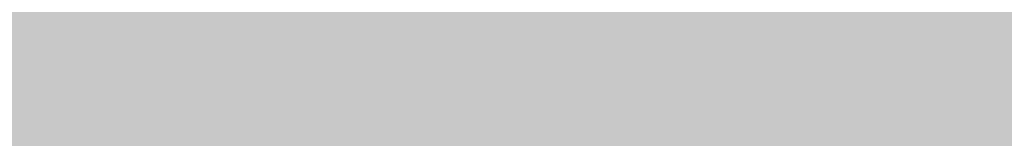
# Model space of a CAD drawing. Units: inches. Extents: x 2083 to 3317, y 1141 to 2115.
# Tile 134 of 256: x 3123.979 to 3126.132, y 1263.355 to 1263.613. Entities that reach past the tile are written whole.
import ezdxf

# ---------------------------------------------------------------- set-up
doc = ezdxf.new("R2010")
doc.units = ezdxf.units.IN
doc.layers.add('A-ANNO-DIMS', color=2, linetype='Continuous', lineweight=18)
doc.layers.add('A-WALL-PATT', color=251, linetype='Continuous', lineweight=13, true_color=0x636466)
doc.styles.get("Standard").update_dxf_attribs({"font": 'arial.ttf'})
doc.dimstyles.new('ISO-25', dxfattribs={"dimtxt": 12, "dimasz": 12, "dimexe": 1.25, "dimexo": 0.625, "dimtad": 1, "dimlunit": 3, "dimtxsty": 'Standard', "dimcen": 2.5, "dimadec": 0, "dimazin": 0, "dimtfac": 1, "dimtmove": 0, "dimatfit": 3, "dimfxl": 1, "dimarcsym": 0})

# ---------------------------------------------------------------- blocks, each defined once
blk = doc.blocks.new('*D26')
at = {"layer": 'A-ANNO-DIMS', "color": 0, "lineweight": -2, "transparency": 16777216}
for p, q in [((3088.9858, 1274.9151), (3088.9858, 1270.952)), ((3111.24, 1274.9151), (3111.24, 1270.952)), ((3076.9858, 1272.202), (2840.2624, 1272.202)), ((3111.24, 1272.202), (3088.9858, 1272.202)), ((3123.24, 1272.202), (3135.24, 1272.202))]:
    blk.add_line(p, q, dxfattribs=at)
at = {"layer": 'A-ANNO-DIMS', "color": 0, "transparency": 16777216}
for points in [[(3076.9858, 1274.202), (3076.9858, 1270.202), (3088.9858, 1272.202)], [(3123.24, 1274.202), (3123.24, 1270.202), (3111.24, 1272.202)]]:
    blk.add_solid(points, dxfattribs=at)
at = {"layer": 'Defpoints', "color": 0, "transparency": 16777216}
for p in [(3088.9858, 1275.5401), (3111.24, 1275.5401), (3088.9858, 1272.202)]:
    blk.add_point(p, dxfattribs=at)
at = {"layer": 'A-ANNO-DIMS', "color": 0, "transparency": 16777216, "insert": (2952.6241, 1279.0316), "char_height": 12, "attachment_point": 5}
blk.add_mtext('NIGHTSTAND 1\'-10 1/2" TYP.', dxfattribs=at)
blk = doc.blocks.new('*D27')
at = {"layer": 'A-ANNO-DIMS', "color": 0, "lineweight": -2, "transparency": 16777216}
for p, q in [((3114.5782, 1309.7943), (3114.5782, 1321.7943)), ((3111.865, 1297.7943), (3115.8282, 1297.7943)), ((3114.5782, 1297.7943), (3114.5782, 1275.5401)), ((3111.865, 1275.5401), (3115.8282, 1275.5401)), ((3114.5782, 1263.5401), (3114.5782, 1140.9886))]:
    blk.add_line(p, q, dxfattribs=at)
at = {"layer": 'A-ANNO-DIMS', "color": 0, "transparency": 16777216}
for points in [[(3112.5782, 1309.7943), (3116.5782, 1309.7943), (3114.5782, 1297.7943)], [(3112.5782, 1263.5401), (3116.5782, 1263.5401), (3114.5782, 1275.5401)]]:
    blk.add_solid(points, dxfattribs=at)
at = {"layer": 'Defpoints', "color": 0, "transparency": 16777216}
for p in [(3111.24, 1297.7943), (3111.24, 1275.5401), (3114.5782, 1275.5401)]:
    blk.add_point(p, dxfattribs=at)
at = {"layer": 'A-ANNO-DIMS', "color": 0, "transparency": 16777216, "insert": (3107.7485, 1196.2643), "char_height": 12, "attachment_point": 5, "rotation": 90}
blk.add_mtext('1\'-10 1/2" TYP.', dxfattribs=at)

msp = doc.modelspace()

# ---------------------------------------------------------------- hatches: boundary and pattern name
at = {"layer": 'A-WALL-PATT'}
h = msp.add_hatch(color=256, dxfattribs=at)
h.dxf.hatch_style = 1
h.paths.add_polyline_path([(3126.9598, 2020.7614), (2748.9598, 2020.7614), (2604.9598, 2020.7614), (2226.9598, 2020.7614), (2226.9598, 1702.7614), (2466.9598, 1702.7614), (2466.9598, 1582.7614), (2418.9598, 1582.7614), (2418.9598, 1477.7614), (2226.9598, 1477.7614), (2226.9598, 1263.2614), (2544.9598, 1263.2614), (2544.9598, 1411.7614), (2604.9598, 1411.7614), (2685.9598, 1411.7614), (2685.9598, 1420.7614), (2604.9598, 1420.7614), (2604.9598, 1573.7614), (2604.9598, 1702.7614), (2604.9598, 2011.7614), (2748.9598, 2011.7614), (2748.9598, 1702.7614), (2862.9598, 1702.7614), (2862.9598, 1621.7614), (2871.9598, 1621.7614), (2871.9598, 1702.7614), (2883.9598, 1702.7614), (2883.9598, 1706.9395, -0.026459), (2883.9598, 1711.7614), (2757.9598, 1711.7614), (2757.9598, 1807.7614), (2787.9598, 1807.7614), (2787.9598, 1812.2614), (2757.9598, 1812.2614), (2757.9598, 2011.7614), (2877.9598, 2011.7614), (2877.9598, 1812.2614), (2847.9598, 1812.2614), (2847.9598, 1807.7614), (2889.8357, 1807.7614), (2889.8357, 1812.2614), (2882.4598, 1812.2614), (2882.4598, 2011.7614), (3117.9598, 2011.7614), (3117.9598, 1812.2614), (2937.8357, 1812.2614), (2937.8357, 1807.7614), (2995.7098, 1807.7614), (2995.7098, 1796.1177), (3000.2098, 1796.1177), (3000.2098, 1807.7614), (3117.9598, 1807.7614), (3117.9598, 1711.7614), (3000.2098, 1711.7614), (3000.2098, 1760.1177), (2998.5727, 1760.1177, -0.020711), (2995.7098, 1760.1177), (2995.7098, 1711.7614), (2931.9598, 1711.7614), (2931.9598, 1702.7614), (3126.9598, 1702.7614)])
h.paths.add_polyline_path([(2471.4598, 2011.7614), (2471.4598, 1810.0114), (2462.7169, 1810.0114), (2462.7169, 1805.5114), (2505.9598, 1805.5114), (2505.9598, 1810.0114), (2475.9598, 1810.0114), (2475.9598, 2011.7614), (2595.9598, 2011.7614), (2595.9598, 1810.0114), (2565.9598, 1810.0114), (2565.9598, 1805.5114), (2595.9598, 1805.5114), (2595.9598, 1711.7614), (2235.9598, 1711.7614), (2235.9598, 1805.5114), (2353.7098, 1805.5114), (2353.7098, 1796.0542), (2358.2098, 1796.0542), (2358.2098, 1805.5114), (2414.7169, 1805.5114), (2414.7169, 1810.0114), (2235.9598, 1810.0114), (2235.9598, 2011.7614)], flags=16)
h.paths.add_polyline_path([(2270.2047, 1994.61), (2270.2047, 1970.61), (2246.2047, 1970.61), (2246.2047, 1994.61)], flags=0)
edge = h.paths.add_edge_path(flags=0)
edge.add_ellipse((2332.0274, 1899.7982), major_axis=(-3.043, 3.043), ratio=0.168252, start_angle=-161.3322, end_angle=-156.3071, ccw=False)
edge.add_ellipse((2333.082, 1898.7435), major_axis=(-1.0546, 1.0546), ratio=0.453532, start_angle=-123.371, end_angle=-94.1591)
edge = h.paths.add_edge_path(flags=0)
edge.add_ellipse((2332.0274, 1968.8763), major_axis=(3.043, 3.043), ratio=0.168252, start_angle=18.6678, end_angle=23.6929)
edge.add_spline(control_points=[(2332.9256, 1970.6911), (2332.2268, 1970.3361), (2330.8937, 1969.6589), (2328.4131, 1970.9321), (2327.2039, 1967.7487), (2324.7096, 1969.9556), (2322.5328, 1967.0124), (2320.0128, 1971.2958), (2317.6803, 1968.1578), (2316.0405, 1967.102), (2315.4269, 1966.8096)], knot_values=[0, 0, 0, 0, 2.267059, 4.324559, 6.685584, 8.878641, 11.121502, 14.300359, 17.755284, 19.732645, 19.732645, 19.732645, 19.732645], degree=3, periodic=0)
edge.add_ellipse((2332.0274, 1968.8763), major_axis=(3.043, 3.043), ratio=0.168252, start_angle=18.6678, end_angle=23.6929, ccw=False)
edge.add_ellipse((2333.082, 1969.9309), major_axis=(1.0546, 1.0546), ratio=0.453532, start_angle=56.629, end_angle=85.8409, ccw=False)
edge = h.paths.add_edge_path(flags=0)
edge.add_spline(control_points=[(2296.4283, 1967.9879), (2293.6278, 1965.3363), (2287.7036, 1959.7271), (2299.7439, 1949.9957), (2294.5326, 1935.6685), (2290.5732, 1920.6035), (2293.3941, 1909.9737), (2296.1854, 1904.9665)], knot_values=[0.099185, 0.099185, 0.099185, 0.099185, 0.345301, 0.619822, 0.982653, 1.386093, 1.810555, 1.810555, 1.810555, 1.810555], degree=3, periodic=0)
edge.add_spline(control_points=[(2296.1854, 1904.9665), (2297.3836, 1902.6193), (2298.001, 1901.9493), (2298.553, 1901.4682)], knot_values=[0.006246, 0.006246, 0.006246, 0.006246, 0.055476, 0.055476, 0.055476, 0.055476], degree=3, periodic=0)
edge.add_spline(control_points=[(2298.553, 1901.4682), (2297.2586, 1900.9232), (2295.2253, 1900.2321), (2293.0602, 1900.6142), (2292.1014, 1900.7884), (2292.0896, 1900.7906)], knot_values=[0.312835, 0.312835, 0.312835, 0.312835, 0.40178, 0.474987, 0.475903, 0.475903, 0.475903, 0.475903], degree=3, periodic=0)
edge.add_arc((2292.7936, 1904.6641), 3.937, 215.4209, 259.6982, ccw=False)
edge.add_spline(control_points=[(2289.5853, 1902.3823), (2289.4767, 1902.5351), (2289.3685, 1902.688), (2289.2609, 1902.8412)], knot_values=[0.102872, 0.102872, 0.102872, 0.102872, 0.116896, 0.116896, 0.116896, 0.116896], degree=3, periodic=0)
edge.add_spline(control_points=[(2289.2609, 1902.8412), (2288.6866, 1902.5502), (2287.64, 1902.0199), (2285.8813, 1901.874), (2283.853, 1901.5044), (2281.72, 1899.7105), (2278.467, 1899.4929), (2276.1571, 1901.8832), (2272.259, 1899.8041), (2267.7776, 1901.8432), (2262.2439, 1900.184), (2257.4149, 1901.7821), (2254.3184, 1900.7261), (2253.1783, 1900.3373)], knot_values=[0, 0, 0, 0, 1.907977, 3.477176, 5.261074, 7.972851, 11.680248, 13.717921, 16.939592, 22.789562, 27.502503, 33.595215, 37.145618, 37.145618, 37.145618, 37.145618], degree=3, periodic=0)
edge.add_line((2253.1783, 1900.3373), (2250.2442, 1902.8412))
edge.add_line((2250.2442, 1902.8412), (2250.2442, 1965.8333))
edge.add_line((2250.2442, 1965.8333), (2253.1783, 1968.3371))
edge.add_spline(control_points=[(2253.1783, 1968.3371), (2254.3184, 1967.9483), (2257.4149, 1966.8924), (2262.2439, 1968.4904), (2267.7776, 1966.8313), (2271.5267, 1968.5372), (2273.8759, 1967.8283), (2274.2067, 1967.7276)], knot_values=[0, 0, 0, 0, 0.09018, 0.244935, 0.364644, 0.513233, 0.537855, 0.537855, 0.537855, 0.537855], degree=3, periodic=0)
edge.add_arc((2274.3529, 1963.7933), 3.937, 72.0511, 92.1279, ccw=False)
edge.add_arc((2281.2969, 1985.23), 18.5963, 252.05113, 288.56572)
edge.add_arc((2292.3167, 1956.0289), 12.6461, 71.02679, 113.77822, ccw=False)
edge = h.paths.add_edge_path(flags=0)
edge.add_spline(control_points=[(2274.8994, 1951.8562), (2275.0662, 1951.6166), (2275.2327, 1951.3766), (2275.398, 1951.1359)], knot_values=[1.409916, 1.409916, 1.409916, 1.409916, 1.43159, 1.43159, 1.43159, 1.43159], degree=3, periodic=0)
edge.add_spline(control_points=[(2275.398, 1951.1359), (2275.7921, 1950.5619), (2276.1792, 1949.9838), (2276.5455, 1949.3971)], knot_values=[1.358238, 1.358238, 1.358238, 1.358238, 1.409916, 1.409916, 1.409916, 1.409916], degree=3, periodic=0)
edge.add_line((2276.5455, 1949.3971), (2277.4373, 1947.8622))
edge.add_spline(control_points=[(2277.4373, 1947.8622), (2276.3038, 1945.6731), (2274.6397, 1942.4269), (2274.6316, 1938.0939), (2272.7991, 1930.8515), (2274.3564, 1943.897), (2275.9477, 1947.9234), (2276.5455, 1949.3971)], knot_values=[0.005632, 0.005632, 0.005632, 0.005632, 0.186014, 0.266002, 0.357087, 0.59639, 0.739732, 0.739732, 0.739732, 0.739732], degree=3, periodic=0)
edge.add_spline(control_points=[(2276.5455, 1949.3971), (2276.1792, 1949.9838), (2275.7921, 1950.5619), (2275.398, 1951.1359)], knot_values=[1.358238, 1.358238, 1.358238, 1.358238, 1.409916, 1.409916, 1.409916, 1.409916], degree=3, periodic=0)
edge.add_spline(control_points=[(2275.398, 1951.1359), (2274.9425, 1950.0805), (2274.2078, 1948.0253), (2273.9346, 1944.8515), (2272.4685, 1937.6275), (2273.4662, 1945.6965), (2274.7006, 1951.0595), (2274.8994, 1951.8562)], knot_values=[0.104364, 0.104364, 0.104364, 0.104364, 0.189636, 0.269624, 0.36071, 0.600013, 0.644622, 0.644622, 0.644622, 0.644622], degree=3, periodic=0)
h.paths.add_polyline_path([(2269.1675, 1963.1276, -0.357527), (2268.1706, 1960.9764, -0.092561), (2268.1706, 1939.4363, -0.357527), (2269.1675, 1937.2851, -0.357527), (2267.0163, 1938.282, -0.164785), (2254.6856, 1938.282, -0.357527), (2252.5344, 1937.2851, -0.357527), (2253.5313, 1939.4363, -0.092561), (2253.5313, 1960.9764, -0.357527), (2252.5344, 1963.1276, -0.357527), (2254.6856, 1962.1307, -0.164785), (2267.0163, 1962.1307, -0.357527)], flags=0)
h.paths.add_polyline_path([(2248.8741, 1967.8018), (2248.8741, 1957.0277), (2249.4578, 1957.0277), (2249.4578, 1911.6468), (2248.8741, 1911.6468), (2248.8741, 1900.8727), (2246.5119, 1900.8727, 0.197327), (2244.1497, 1902.4569), (2244.1497, 1966.2176, 0.197327), (2246.5119, 1967.8018)], flags=0)
h.paths.add_polyline_path([(2269.1675, 1931.3893, -0.357527), (2268.1706, 1929.2381, -0.092561), (2268.1706, 1907.6981, -0.357527), (2269.1675, 1905.5469, -0.357527), (2267.0163, 1906.5438, -0.164785), (2254.6856, 1906.5438, -0.357527), (2252.5344, 1905.5469, -0.357527), (2253.5313, 1907.6981, -0.092561), (2253.5313, 1929.2381, -0.357527), (2252.5344, 1931.3893, -0.357527), (2254.6856, 1930.3925, -0.164785), (2267.0163, 1930.3925, -0.357527)], flags=0)
edge = h.paths.add_edge_path(flags=0)
edge.add_spline(control_points=[(2276.1969, 1906.7237), (2276.1681, 1909.0289), (2276.114, 1913.3719), (2270.5984, 1924.925), (2273.9052, 1919.0128), (2275.9217, 1916.2621), (2275.4746, 1912.4021), (2277.2579, 1910.3806), (2276.696, 1908.225), (2276.6462, 1906.813), (2276.6178, 1906.0084)], knot_values=[0, 0, 0, 0, 8.61026, 16.221274, 18.843057, 23.804898, 27.440828, 29.356102, 31.203478, 33.650687, 33.650687, 33.650687, 33.650687], degree=3, periodic=0)
edge.add_spline(control_points=[(2276.6178, 1906.0084), (2276.6233, 1905.6241), (2276.4977, 1904.6287), (2275.4418, 1903.8547), (2274.9373, 1903.0804), (2274.8591, 1902.8412)], knot_values=[0.156488, 0.156488, 0.156488, 0.156488, 0.184398, 0.231376, 0.250598, 0.250598, 0.250598, 0.250598], degree=3, periodic=0)
edge.add_line((2274.8591, 1902.8412), (2276.506, 1902.8412))
edge.add_spline(control_points=[(2276.506, 1902.8412), (2276.7883, 1903.0849), (2277.6651, 1904.1252), (2278.2495, 1904.3407), (2277.6539, 1908.5274), (2278.1557, 1906.2278), (2278.1005, 1905.2859), (2278.8467, 1904.069), (2277.8568, 1903.4149), (2277.8742, 1902.991), (2277.9036, 1902.8412)], knot_values=[0.059574, 0.059574, 0.059574, 0.059574, 0.080753, 0.103741, 0.16972, 0.176036, 0.207137, 0.240474, 0.262341, 0.27366, 0.27366, 0.27366, 0.27366], degree=3, periodic=0)
edge.add_line((2277.9036, 1902.8412), (2280.0298, 1902.8412))
edge.add_spline(control_points=[(2280.0298, 1902.8412), (2279.8882, 1903.0884), (2279.4993, 1903.9816), (2280.1523, 1905.9393), (2278.1036, 1909.6578), (2279.7624, 1907.1853), (2280.3279, 1904.8749), (2280.4851, 1903.4896), (2281.4633, 1903.2494), (2281.7583, 1902.9365), (2281.834, 1902.8412)], knot_values=[0.013856, 0.013856, 0.013856, 0.013856, 0.034874, 0.088867, 0.107879, 0.126738, 0.158714, 0.193757, 0.217487, 0.226722, 0.226722, 0.226722, 0.226722], degree=3, periodic=0)
edge.add_spline(control_points=[(2281.834, 1902.8412), (2281.7875, 1902.8267), (2281.647, 1902.783), (2281.3955, 1902.8595), (2281.0881, 1902.9852), (2280.7207, 1903.0609), (2280.3335, 1903.0257), (2280.1248, 1902.8989), (2280.0298, 1902.8412)], knot_values=[0, 0, 0, 0, 0.14413, 0.435517, 0.749276, 1.153046, 1.548371, 1.878348, 1.878348, 1.878348, 1.878348], degree=3, periodic=0)
edge.add_line((2280.0298, 1902.8412), (2277.9036, 1902.8412))
edge.add_spline(control_points=[(2277.9036, 1902.8412), (2277.8929, 1902.7959), (2277.8654, 1902.6796), (2277.6075, 1902.6875), (2277.2741, 1902.8007), (2276.8379, 1902.6198), (2276.5838, 1902.7893), (2276.506, 1902.8412)], knot_values=[0, 0, 0, 0, 0.127189, 0.326199, 0.628009, 1.24357, 1.515331, 1.515331, 1.515331, 1.515331], degree=3, periodic=0)
edge.add_line((2276.506, 1902.8412), (2274.8591, 1902.8412))
edge.add_spline(control_points=[(2274.8591, 1902.8412), (2274.8144, 1902.8986), (2274.7251, 1903.0134), (2274.4935, 1903.119), (2274.2443, 1902.9605), (2273.9371, 1903.1849), (2273.614, 1902.9831), (2273.4083, 1902.883), (2273.3223, 1902.8412)], knot_values=[0, 0, 0, 0, 0.21843, 0.436957, 0.687977, 0.990379, 1.398396, 1.69185, 1.69185, 1.69185, 1.69185], degree=3, periodic=0)
edge.add_spline(control_points=[(2273.3223, 1902.8412), (2273.6167, 1903.4457), (2274.274, 1904.5383), (2276.0272, 1904.5737), (2276.207, 1906.5836), (2276.1969, 1906.7237)], knot_values=[0.012227, 0.012227, 0.012227, 0.012227, 0.059472, 0.106218, 0.134458, 0.134458, 0.134458, 0.134458], degree=3, periodic=0)
h.paths.add_polyline_path([(2270.7761, 1897.7898), (2270.7761, 1873.7898), (2246.7761, 1873.7898), (2246.7761, 1897.7898)], flags=0)
h.paths.add_polyline_path([(2353.7098, 1760.0051), (2353.7098, 1760.0542), (2358.2098, 1760.0542, -0.033729)], flags=0)
h.paths.add_polyline_path([(2321.8191, 1737.5292), (2341.9953, 1737.5292, -0.414214), (2343.2033, 1736.3212), (2343.2033, 1721.0206, -0.414214), (2341.9953, 1719.8127), (2321.8191, 1719.8127, -0.414214), (2320.6112, 1721.0206), (2320.6112, 1736.3212, -0.414214)], flags=0)
h.paths.add_polyline_path([(2324.235, 1736.3212), (2339.5794, 1736.3212, -0.414214), (2341.9953, 1733.9053), (2341.9953, 1725.4497, -0.414214), (2339.5794, 1723.0338), (2333.6806, 1723.0338), (2333.8453, 1722.0455, -0.870646), (2335.4254, 1721.8259, -0.767327), (2333.9227, 1721.4232), (2331.291, 1721.4232, -0.767327), (2329.7883, 1721.8259, -0.870646), (2331.3684, 1722.0455), (2331.5331, 1723.0338), (2324.235, 1723.0338, -0.414214), (2321.8191, 1725.4497), (2321.8191, 1733.9053, -0.414214)], flags=0)
h.paths.add_polyline_path([(2570.4838, 1928.6154), (2589.6838, 1928.6154), (2590.1688, 1928.6154), (2590.1688, 1904.9934), (2570.4838, 1904.9934)], flags=0)
h.paths.add_polyline_path([(2574.4473, 1927.2638, -1), (2572.8288, 1927.2638, -1)], flags=0)
h.paths.add_polyline_path([(2573.0899, 1926.9409), (2573.925, 1927.776), (2574.1477, 1927.5533), (2573.3126, 1926.7182)], flags=0)
h.paths.add_polyline_path([(2578.7791, 1919.7296, -1), (2571.5917, 1919.7296, -1)], flags=0)
h.paths.add_polyline_path([(2578.3854, 1919.7296, -1), (2571.9854, 1919.7296, -1)], flags=0)
h.paths.add_polyline_path([(2331.5958, 1729.4762, -1), (2333.618, 1729.4762, -1)], flags=0)
h.paths.add_polyline_path([(2578.0342, 1927.2638, -1), (2576.4157, 1927.2638, -1)], flags=0)
h.paths.add_polyline_path([(2576.6889, 1927.5311), (2576.9116, 1927.7538), (2577.7467, 1926.9186), (2577.524, 1926.6959)], flags=0)
h.paths.add_polyline_path([(2578.1391, 1909.8595, -1), (2572.2317, 1909.8595, -1)], flags=0)
h.paths.add_polyline_path([(2577.7454, 1909.8595, -1), (2572.6254, 1909.8595, -1)], flags=0)
h.paths.add_polyline_path([(2583.7977, 1927.2638, -1), (2582.1792, 1927.2638, -1)], flags=0)
h.paths.add_polyline_path([(2582.7186, 1927.7538), (2583.5538, 1926.9186), (2583.3311, 1926.6959), (2582.4959, 1927.5311)], flags=0)
h.paths.add_polyline_path([(2582.4959, 1927.5311), (2582.7186, 1927.7538), (2583.5538, 1926.9186), (2583.3311, 1926.6959)], flags=0)
h.paths.add_polyline_path([(2587.7391, 1920.5296, -1), (2581.8317, 1920.5296, -1)], flags=0)
h.paths.add_polyline_path([(2587.3454, 1920.5296, -1), (2582.2254, 1920.5296, -1)], flags=0)
h.paths.add_polyline_path([(2587.3846, 1927.2638, -1), (2585.7661, 1927.2638, -1)], flags=0)
h.paths.add_polyline_path([(2586.082, 1926.9802), (2586.9172, 1927.8154), (2587.1399, 1927.5927), (2586.3047, 1926.7575)], flags=0)
h.paths.add_polyline_path([(2588.3791, 1910.6595, -1), (2581.1917, 1910.6595, -1)], flags=0)
h.paths.add_polyline_path([(2587.9854, 1910.6595, -1), (2581.5854, 1910.6595, -1)], flags=0)
h.paths.add_polyline_path([(2417.1677, 1729.4779), (2437.3439, 1729.4779, -0.414214), (2438.5519, 1728.2699), (2438.5519, 1712.9693, -0.414214), (2437.3439, 1711.7614), (2417.1677, 1711.7614, -0.414214), (2415.9598, 1712.9693), (2415.9598, 1728.2699, -0.414214)], flags=0)
h.paths.add_polyline_path([(2419.5836, 1728.2699), (2434.928, 1728.2699, -0.414214), (2437.3439, 1725.8541), (2437.3439, 1717.3984, -0.414214), (2434.928, 1714.9825), (2429.0292, 1714.9825), (2429.1939, 1713.9942, -0.870646), (2430.774, 1713.7746, -0.767327), (2429.2713, 1713.372), (2426.6396, 1713.372, -0.767327), (2425.1369, 1713.7746, -0.870646), (2426.717, 1713.9942), (2426.8817, 1714.9825), (2419.5836, 1714.9825, -0.414214), (2417.1677, 1717.3984), (2417.1677, 1725.8541, -0.414214)], flags=0)
h.paths.add_polyline_path([(2419.5836, 1728.2699), (2434.928, 1728.2699, -0.414214), (2437.3439, 1725.8541), (2437.3439, 1717.3984, -0.414214), (2434.928, 1714.9825), (2429.0292, 1714.9825), (2428.3581, 1719.009), (2427.5528, 1719.009), (2426.8817, 1714.9825), (2419.5836, 1714.9825, -0.414214), (2417.1677, 1717.3984), (2417.1677, 1725.8541, -0.414214)], flags=0)
h.paths.add_polyline_path([(2426.9444, 1721.4249, -1), (2428.9666, 1721.4249, -1)], flags=0)
h.paths.add_polyline_path([(2475.9598, 1702.7614), (2595.9598, 1702.7614), (2595.9598, 1582.7614), (2475.9598, 1582.7614)], flags=16)
h.paths.add_polyline_path([(2427.9598, 1573.7614), (2595.9598, 1573.7614), (2595.9598, 1468.7614), (2595.9598, 1420.7614), (2384.4598, 1420.7614), (2384.4598, 1468.7614), (2427.9598, 1468.7614)], flags=16)
h.paths.add_polyline_path([(2379.9598, 1468.7614), (2379.9598, 1420.7614), (2235.9598, 1420.7614), (2235.9598, 1468.7614)], flags=16)
h.paths.add_polyline_path([(2317.816, 1466.6958), (2337.9922, 1466.6958, -0.414214), (2339.2002, 1465.4878), (2339.2002, 1450.1872, -0.414214), (2337.9922, 1448.9792), (2317.816, 1448.9792, -0.414214), (2316.6081, 1450.1872), (2316.6081, 1465.4878, -0.414214)], flags=0)
h.paths.add_polyline_path([(2320.2319, 1465.4878), (2335.5763, 1465.4878, -0.414214), (2337.9922, 1463.0719), (2337.9922, 1454.6163, -0.414214), (2335.5763, 1452.2004), (2329.6775, 1452.2004), (2329.8422, 1451.212, -0.870646), (2331.4223, 1450.9925, -0.767327), (2329.9196, 1450.5898), (2327.2879, 1450.5898, -0.767327), (2325.7852, 1450.9925, -0.870646), (2327.3653, 1451.212), (2327.53, 1452.2004), (2320.2319, 1452.2004, -0.414214), (2317.816, 1454.6163), (2317.816, 1463.0719, -0.414214)], flags=0)
h.paths.add_polyline_path([(2320.2319, 1465.4878), (2335.5763, 1465.4878, -0.414214), (2337.9922, 1463.0719), (2337.9922, 1454.6163, -0.414214), (2335.5763, 1452.2004), (2329.6775, 1452.2004), (2329.0064, 1456.2269), (2328.2011, 1456.2269), (2327.53, 1452.2004), (2320.2319, 1452.2004, -0.414214), (2317.816, 1454.6163), (2317.816, 1463.0719, -0.414214)], flags=0)
h.paths.add_polyline_path([(2327.5926, 1458.6428, -1), (2329.6148, 1458.6428, -1)], flags=0)
h.paths.add_polyline_path([(2244.4117, 1433.3405), (2241.9209, 1433.3405, -0.414214), (2240.0179, 1435.2435), (2240.0179, 1440.9528, -0.414211), (2241.9209, 1442.8559), (2244.4117, 1442.8559, -1.976472)], flags=0)
h.paths.add_polyline_path([(2245.3569, 1434.3975, -0.414214), (2245.3569, 1441.7988, -2.144098)], flags=0)
h.paths.add_polyline_path([(2535.9598, 1416.2614), (2535.9598, 1272.2614), (2235.9598, 1272.2614), (2235.9598, 1416.2614)], flags=16)
h.paths.add_polyline_path([(2260.1196, 1384.2928), (2260.1196, 1362.0386), (2237.8654, 1362.0386), (2237.8654, 1384.2928)], flags=0)
edge = h.paths.add_edge_path(flags=0)
edge.add_line((2318.2518, 1362.0933), (2318.1458, 1362.001))
edge.add_ellipse((2317.4451, 1360.431), major_axis=(2.8216, 2.8216), ratio=0.168252, start_angle=18.6678, end_angle=20.9481, ccw=False)
edge.add_ellipse((2318.423, 1361.409), major_axis=(0.9779, 0.9779), ratio=0.453532, start_angle=56.629, end_angle=70.2262, ccw=False)
edge = h.paths.add_edge_path(flags=0)
edge.add_line((2319.1074, 1295.5711), (2319.015, 1295.6771))
edge.add_ellipse((2317.4451, 1296.3778), major_axis=(-2.8216, 2.8216), ratio=0.168252, start_angle=-161.3322, end_angle=-159.0519, ccw=False)
edge.add_ellipse((2318.423, 1295.3999), major_axis=(-0.9779, 0.9779), ratio=0.453532, start_angle=-123.371, end_angle=-109.7738)
edge = h.paths.add_edge_path(flags=0)
edge.add_spline(control_points=[(2284.2103, 1301.1702), (2284.5807, 1300.4447), (2284.8912, 1299.892), (2285.1596, 1299.461)], knot_values=[0.039066, 0.039066, 0.039066, 0.039066, 0.055476, 0.055476, 0.055476, 0.055476], degree=3, periodic=0)
edge.add_line((2285.1596, 1299.461), (2284.2103, 1301.1702))
edge = h.paths.add_edge_path(flags=0)
edge.add_line((2280.4125, 1297.298), (2283.37, 1297.0361))
edge.add_line((2283.37, 1297.0361), (2286.4057, 1297.9263))
edge.add_spline(control_points=[(2286.4057, 1297.9263), (2285.3055, 1297.4631), (2284.3448, 1297.1292), (2283.37, 1297.0361)], knot_values=[0.394369, 0.394369, 0.394369, 0.394369, 0.475903, 0.475903, 0.475903, 0.475903], degree=3, periodic=0)
edge.add_spline(control_points=[(2283.37, 1297.0361), (2283.2814, 1297.0277), (2282.3163, 1296.9573), (2281.3125, 1297.1345), (2280.4234, 1297.296), (2280.4125, 1297.298)], knot_values=[0.312835, 0.312835, 0.312835, 0.312835, 0.320246, 0.393453, 0.394369, 0.394369, 0.394369, 0.394369], degree=3, periodic=0)
edge = h.paths.add_edge_path(flags=0)
edge.add_line((2284.4356, 1359.6073), (2280.4463, 1355.328))
edge.add_line((2280.4463, 1355.328), (2279.58, 1351.0178))
edge.add_line((2279.58, 1351.0178), (2282.413, 1346.5804))
edge.add_spline(control_points=[(2282.413, 1346.5804), (2283.1533, 1345.5892), (2284.2529, 1344.0289), (2284.801, 1342.3872), (2284.9352, 1341.8055)], knot_values=[1.240098, 1.240098, 1.240098, 1.240098, 1.332892, 1.382712, 1.382712, 1.382712, 1.382712], degree=3, periodic=0)
edge.add_spline(control_points=[(2284.9352, 1341.8055), (2285.3191, 1340.1406), (2285.233, 1338.4092), (2284.9099, 1336.6541)], knot_values=[1.097484, 1.097484, 1.097484, 1.097484, 1.240098, 1.240098, 1.240098, 1.240098], degree=3, periodic=0)
edge.add_spline(control_points=[(2284.9099, 1336.6541), (2284.5868, 1334.899), (2284.0267, 1333.1203), (2283.4626, 1331.3606)], knot_values=[0.95487, 0.95487, 0.95487, 0.95487, 1.097484, 1.097484, 1.097484, 1.097484], degree=3, periodic=0)
edge.add_line((2283.4626, 1331.3606), (2281.8904, 1326.1534))
edge.add_line((2281.8904, 1326.1534), (2280.7563, 1321.0561))
edge.add_line((2280.7563, 1321.0561), (2280.2992, 1316.002))
edge.add_line((2280.2992, 1316.002), (2280.7159, 1310.9501))
edge.add_line((2280.7159, 1310.9501), (2282.0281, 1305.9721))
edge.add_line((2282.0281, 1305.9721), (2284.2103, 1301.1702))
edge.add_spline(control_points=[(2284.2103, 1301.1702), (2283.3407, 1302.7302), (2282.6119, 1304.3365), (2282.0281, 1305.9721)], knot_values=[0.099185, 0.099185, 0.099185, 0.099185, 0.241799, 0.241799, 0.241799, 0.241799], degree=3, periodic=0)
edge.add_spline(control_points=[(2282.0281, 1305.9721), (2281.4443, 1307.6078), (2281.0055, 1309.2728), (2280.7159, 1310.9501)], knot_values=[0.241799, 0.241799, 0.241799, 0.241799, 0.384413, 0.384413, 0.384413, 0.384413], degree=3, periodic=0)
edge.add_spline(control_points=[(2280.7159, 1310.9501), (2280.4332, 1312.5876), (2280.2894, 1314.277), (2280.2989, 1315.962), (2280.2992, 1316.002)], knot_values=[0.384413, 0.384413, 0.384413, 0.384413, 0.523647, 0.527028, 0.527028, 0.527028, 0.527028], degree=3, periodic=0)
edge.add_spline(control_points=[(2280.2992, 1316.002), (2280.3123, 1317.687), (2280.4779, 1319.3679), (2280.7563, 1321.0561)], knot_values=[0.527028, 0.527028, 0.527028, 0.527028, 0.669642, 0.669642, 0.669642, 0.669642], degree=3, periodic=0)
edge.add_spline(control_points=[(2280.7563, 1321.0561), (2281.0346, 1322.7443), (2281.4259, 1324.4396), (2281.8904, 1326.1534)], knot_values=[0.669642, 0.669642, 0.669642, 0.669642, 0.812256, 0.812256, 0.812256, 0.812256], degree=3, periodic=0)
edge.add_spline(control_points=[(2281.8904, 1326.1534), (2282.2644, 1327.5333), (2282.7879, 1329.2618), (2283.3528, 1331.0178), (2283.4626, 1331.3606)], knot_values=[0.812256, 0.812256, 0.812256, 0.812256, 0.927087, 0.95487, 0.95487, 0.95487, 0.95487], degree=3, periodic=0)
edge.add_line((2283.4626, 1331.3606), (2284.9099, 1336.6541))
edge.add_line((2284.9099, 1336.6541), (2284.9352, 1341.8055))
edge.add_line((2284.9352, 1341.8055), (2282.413, 1346.5804))
edge.add_spline(control_points=[(2282.413, 1346.5804), (2281.2751, 1348.1038), (2280.0784, 1349.5703), (2279.58, 1351.0178)], knot_values=[1.382712, 1.382712, 1.382712, 1.382712, 1.525326, 1.525326, 1.525326, 1.525326], degree=3, periodic=0)
edge.add_spline(control_points=[(2279.58, 1351.0178), (2279.4433, 1351.4147), (2279.1363, 1352.8569), (2279.7352, 1354.2904), (2280.4463, 1355.328)], knot_values=[1.525326, 1.525326, 1.525326, 1.525326, 1.564439, 1.667941, 1.667941, 1.667941, 1.667941], degree=3, periodic=0)
edge.add_spline(control_points=[(2280.4463, 1355.328), (2281.4261, 1356.7578), (2282.9308, 1358.1826), (2284.4356, 1359.6073)], knot_values=[1.667941, 1.667941, 1.667941, 1.667941, 1.810555, 1.810555, 1.810555, 1.810555], degree=3, periodic=0)
edge.add_arc((2280.6231, 1348.5182), 11.7262, 71.02679, 113.77822)
edge.add_arc((2270.4049, 1375.5952), 17.2436, 252.05113, 288.56572, ccw=False)
edge.add_arc((2263.966, 1355.7178), 3.6506, 72.0511, 92.1279)
edge.add_arc((2263.966, 1355.7178), 3.6506, 92.1279, 177.9851)
edge.add_spline(control_points=[(2260.3176, 1355.8462), (2260.2604, 1354.2207), (2260.5513, 1350.1865), (2262.9993, 1346.7663), (2264.4727, 1344.649)], knot_values=[1.43159, 1.43159, 1.43159, 1.43159, 1.564144, 1.770695, 1.770695, 1.770695, 1.770695], degree=3, periodic=0)
edge.add_line((2264.4727, 1344.649), (2264.9356, 1343.9825))
edge.add_spline(control_points=[(2263.801, 1340.2481), (2263.8432, 1340.5141), (2264.0672, 1341.7565), (2264.5127, 1343.0025), (2264.935, 1343.9811)], knot_values=[0.53657, 0.53657, 0.53657, 0.53657, 0.559349, 0.644622, 0.644622, 0.644622, 0.644622], degree=3, periodic=0)
edge.add_spline(control_points=[(2264.935, 1343.9811), (2265.1178, 1343.715), (2265.2989, 1343.4479), (2265.4768, 1343.1794)], knot_values=[1.384077, 1.384077, 1.384077, 1.384077, 1.409916, 1.409916, 1.409916, 1.409916], degree=3, periodic=0)
edge.add_spline(control_points=[(2265.4768, 1343.1794), (2265.6546, 1342.9108), (2265.8293, 1342.6408), (2265.9991, 1342.3688)], knot_values=[1.358238, 1.358238, 1.358238, 1.358238, 1.384077, 1.384077, 1.384077, 1.384077], degree=3, periodic=0)
edge.add_line((2265.9991, 1342.3688), (2266.826, 1340.9455))
edge.add_spline(control_points=[(2266.826, 1340.9455), (2268.8944, 1337.0897), (2271.3982, 1325.843), (2270.5162, 1310.5686), (2275.9194, 1301.8606), (2277.7895, 1299.1994)], knot_values=[0.116896, 0.116896, 0.116896, 0.116896, 0.472987, 1.050969, 1.313793, 1.313793, 1.313793, 1.313793], degree=3, periodic=0)
edge.add_spline(control_points=[(2277.7895, 1299.1994), (2277.8394, 1299.1285), (2277.8894, 1299.0575), (2277.9396, 1298.9866)], knot_values=[0.109884, 0.109884, 0.109884, 0.109884, 0.116896, 0.116896, 0.116896, 0.116896], degree=3, periodic=0)
edge.add_line((2277.9396, 1298.9866), (2277.7888, 1299.1991))
edge.add_spline(control_points=[(2277.7888, 1299.1991), (2277.2566, 1298.9294), (2276.2864, 1298.4379), (2275.0394, 1298.3344), (2274.3833, 1298.2389), (2274.2153, 1298.2093)], knot_values=[33.12187, 33.12187, 33.12187, 33.12187, 35.029056, 36.598255, 37.144827, 37.144827, 37.144827, 37.144827], degree=3, periodic=0)
edge.add_line((2274.2153, 1298.2093), (2273.0731, 1297.893))
edge.add_spline(control_points=[(2273.0731, 1297.893), (2272.3229, 1297.5798), (2271.0392, 1296.5105), (2269.2484, 1296.2261), (2268.4231, 1296.3747)], knot_values=[26.532584, 26.532584, 26.532584, 26.532584, 29.198919, 31.839101, 31.839101, 31.839101, 31.839101], degree=3, periodic=0)
edge.add_line((2268.4231, 1296.3747), (2263.8785, 1297.4575))
edge.add_spline(control_points=[(2263.8785, 1297.4575), (2263.5561, 1297.3594), (2261.8603, 1296.8387), (2260.2388, 1297.2824), (2258.9335, 1297.5165)], knot_values=[15.919551, 15.919551, 15.919551, 15.919551, 16.939592, 21.226067, 21.226067, 21.226067, 21.226067], degree=3, periodic=0)
edge.add_line((2258.9335, 1297.5165), (2254.0552, 1297.329))
edge.add_spline(control_points=[(2254.0552, 1297.329), (2253.7555, 1297.2958), (2252.1137, 1297.1652), (2250.4619, 1297.5442), (2249.1297, 1297.6679)], knot_values=[5.306517, 5.306517, 5.306517, 5.306517, 6.276435, 10.613034, 10.613034, 10.613034, 10.613034], degree=3, periodic=0)
edge.add_line((2249.1297, 1297.6679), (2244.3316, 1296.8778))
edge.add_line((2244.3316, 1296.8778), (2241.611, 1299.1994))
edge.add_line((2241.611, 1299.1994), (2241.611, 1357.6094))
edge.add_line((2241.611, 1357.6094), (2244.3316, 1359.9311))
edge.add_line((2244.3316, 1359.9311), (2252.7288, 1359.5427))
edge.add_spline(control_points=[(2252.7288, 1359.5427), (2252.8709, 1359.5464), (2253.3057, 1359.5482), (2253.7398, 1359.5143), (2254.0317, 1359.4824)], knot_values=[0.233291, 0.233291, 0.233291, 0.233291, 0.244935, 0.268927, 0.268927, 0.268927, 0.268927], degree=3, periodic=0)
edge.add_line((2254.0317, 1359.4824), (2259.5872, 1359.4164))
edge.add_spline(control_points=[(2259.5872, 1359.4164), (2260.6771, 1359.6285), (2262.0732, 1359.897), (2263.5237, 1359.4593), (2263.8304, 1359.366)], knot_values=[0.422516, 0.422516, 0.422516, 0.422516, 0.513233, 0.537855, 0.537855, 0.537855, 0.537855], degree=3, periodic=0)
edge.add_arc((2263.966, 1355.7178), 3.6506, 72.0511, 92.1279, ccw=False)
edge.add_arc((2270.4049, 1375.5952), 17.2436, 252.05113, 288.56572)
edge.add_arc((2280.6231, 1348.5182), 11.7262, 71.02679, 113.77822, ccw=False)
h.paths.add_polyline_path([(2240.3405, 1359.4347), (2240.3405, 1349.4444), (2240.8818, 1349.4444), (2240.8818, 1307.3645), (2240.3405, 1307.3645), (2240.3405, 1297.3741), (2238.1502, 1297.3741, 0.197327), (2235.9598, 1298.8431), (2235.9598, 1357.9657, 0.197327), (2238.1502, 1359.4347)], flags=0)
h.paths.add_polyline_path([(2259.1578, 1355.1005, -0.357527), (2258.2334, 1353.1058, -0.092561), (2258.2334, 1333.1326, -0.357527), (2259.1578, 1331.1379, -0.357527), (2257.1631, 1332.0622, -0.164785), (2245.7293, 1332.0622, -0.357527), (2243.7346, 1331.1379, -0.357527), (2244.6589, 1333.1326, -0.092561), (2244.6589, 1353.1058, -0.357527), (2243.7346, 1355.1005, -0.357527), (2245.7293, 1354.1761, -0.164785), (2257.1631, 1354.1761, -0.357527)], flags=0)
edge = h.paths.add_edge_path(flags=0)
edge.add_line((2265.9991, 1342.3688), (2266.826, 1340.9455))
edge.add_line((2266.826, 1340.9455), (2265.3076, 1337.8141))
edge.add_line((2265.3076, 1337.8141), (2264.3582, 1334.6529))
edge.add_line((2264.3582, 1334.6529), (2264.262, 1333.7997))
edge.add_spline(control_points=[(2264.262, 1333.7997), (2264.2084, 1333.1871), (2264.1621, 1332.3655), (2264.0071, 1331.4139), (2263.969, 1331.2018)], knot_values=[0.464444, 0.464444, 0.464444, 0.464444, 0.516691, 0.531608, 0.531608, 0.531608, 0.531608], degree=3, periodic=0)
edge.add_spline(control_points=[(2263.969, 1331.2018), (2263.7745, 1330.1189), (2263.4244, 1328.7908), (2263.2574, 1328.5307), (2263.234, 1328.5146)], knot_values=[0.372682, 0.372682, 0.372682, 0.372682, 0.44885, 0.464444, 0.464444, 0.464444, 0.464444], degree=3, periodic=0)
edge.add_spline(control_points=[(2263.234, 1328.5146), (2263.0964, 1328.4202), (2263.1312, 1329.3015), (2263.275, 1330.6157)], knot_values=[0.280919, 0.280919, 0.280919, 0.280919, 0.372682, 0.372682, 0.372682, 0.372682], degree=3, periodic=0)
edge.add_spline(control_points=[(2263.275, 1330.6157), (2263.4187, 1331.93), (2263.6715, 1333.6773), (2263.9699, 1335.315)], knot_values=[0.189157, 0.189157, 0.189157, 0.189157, 0.280919, 0.280919, 0.280919, 0.280919], degree=3, periodic=0)
edge.add_spline(control_points=[(2263.9699, 1335.315), (2264.1005, 1336.0322), (2264.4188, 1337.6219), (2264.7548, 1338.8644), (2264.9474, 1339.4911)], knot_values=[0.097394, 0.097394, 0.097394, 0.097394, 0.137578, 0.189157, 0.189157, 0.189157, 0.189157], degree=3, periodic=0)
edge.add_spline(control_points=[(2264.9474, 1339.4911), (2265.29, 1340.6061), (2265.6442, 1341.494), (2265.9991, 1342.3688)], knot_values=[0.005632, 0.005632, 0.005632, 0.005632, 0.097394, 0.097394, 0.097394, 0.097394], degree=3, periodic=0)
h.paths.add_polyline_path([(2259.1578, 1325.671, -0.357527), (2258.2334, 1323.6763, -0.092561), (2258.2334, 1303.7031, -0.357527), (2259.1578, 1301.7084, -0.357527), (2257.1631, 1302.6327, -0.164785), (2245.7293, 1302.6327, -0.357527), (2243.7346, 1301.7084, -0.357527), (2244.6589, 1303.7031, -0.092561), (2244.6589, 1323.6763, -0.357527), (2243.7346, 1325.671, -0.357527), (2245.7293, 1324.7466, -0.164785), (2257.1631, 1324.7466, -0.357527)], flags=0)
edge = h.paths.add_edge_path(flags=0)
edge.add_spline(control_points=[(2261.7089, 1317.3114), (2261.6795, 1317.4176), (2261.7619, 1317.3885), (2262.4907, 1316.0899), (2262.9622, 1315.3009)], knot_values=[14.955861, 14.955861, 14.955861, 14.955861, 16.221274, 18.694826, 18.694826, 18.694826, 18.694826], degree=3, periodic=0)
edge.add_spline(control_points=[(2262.9622, 1315.3009), (2262.9904, 1315.2536), (2263.7021, 1314.0674), (2264.349, 1313.1272), (2264.7301, 1312.1642)], knot_values=[18.694826, 18.694826, 18.694826, 18.694826, 18.843057, 22.433791, 22.433791, 22.433791, 22.433791], degree=3, periodic=0)
edge.add_spline(control_points=[(2264.7301, 1312.1642), (2264.8756, 1311.7964), (2265.1769, 1310.7698), (2265.1431, 1309.5593), (2265.2477, 1308.8242)], knot_values=[22.433791, 22.433791, 22.433791, 22.433791, 23.804898, 26.172756, 26.172756, 26.172756, 26.172756], degree=3, periodic=0)
edge.add_line((2265.2477, 1308.8242), (2265.8508, 1307.1719))
edge.add_spline(control_points=[(2265.8508, 1307.1719), (2266.065, 1306.8217), (2266.3844, 1306.3322), (2266.4244, 1305.7805), (2266.4204, 1305.6112)], knot_values=[28.062562, 28.062562, 28.062562, 28.062562, 29.356102, 29.911721, 29.911721, 29.911721, 29.911721], degree=3, periodic=0)
edge.add_spline(control_points=[(2266.4204, 1305.6112), (2266.4161, 1305.4326), (2266.394, 1305.25), (2266.3648, 1305.0659)], knot_values=[29.911721, 29.911721, 29.911721, 29.911721, 30.497837, 30.497837, 30.497837, 30.497837], degree=3, periodic=0)
edge.add_line((2266.3648, 1305.0659), (2266.0662, 1302.1363))
edge.add_spline(control_points=[(2266.0662, 1302.1363), (2266.0712, 1301.78), (2265.9981, 1301.2), (2265.6633, 1300.759), (2265.5089, 1300.5859)], knot_values=[0.156488, 0.156488, 0.156488, 0.156488, 0.184398, 0.203543, 0.203543, 0.203543, 0.203543], degree=3, periodic=0)
edge.add_line((2265.5089, 1300.5859), (2264.4353, 1299.1994))
edge.add_line((2264.4353, 1299.1994), (2265.9624, 1299.1994))
edge.add_line((2265.9624, 1299.1994), (2267.336, 1301.1753))
edge.add_line((2267.336, 1301.1753), (2267.3117, 1301.9862))
edge.add_spline(control_points=[(2267.3117, 1301.9862), (2267.2611, 1302.8624), (2267.1602, 1303.7371), (2267.2715, 1303.3259)], knot_values=[0.126229, 0.126229, 0.126229, 0.126229, 0.166617, 0.166617, 0.166617, 0.166617], degree=3, periodic=0)
edge.add_spline(control_points=[(2267.2715, 1303.3259), (2267.28, 1303.2943), (2267.3098, 1303.1754), (2267.3735, 1302.8836), (2267.4061, 1302.6828), (2267.4179, 1302.601)], knot_values=[0.166617, 0.166617, 0.166617, 0.166617, 0.16972, 0.176036, 0.180765, 0.180765, 0.180765, 0.180765], degree=3, periodic=0)
edge.add_spline(control_points=[(2267.7439, 1300.9875), (2267.6876, 1301.1509), (2267.4805, 1301.6567), (2267.4838, 1302.1448), (2267.4179, 1302.601)], knot_values=[0.180765, 0.180765, 0.180765, 0.180765, 0.193767, 0.220139, 0.220139, 0.220139, 0.220139], degree=3, periodic=0)
edge.add_line((2267.4179, 1302.601), (2267.7439, 1300.9875))
edge.add_spline(control_points=[(2267.7439, 1300.9875), (2267.832, 1300.7319), (2267.932, 1300.3099), (2267.5548, 1299.9745), (2267.4294, 1299.8292)], knot_values=[0.220139, 0.220139, 0.220139, 0.220139, 0.240474, 0.25489, 0.25489, 0.25489, 0.25489], degree=3, periodic=0)
edge.add_line((2267.4294, 1299.8292), (2267.2584, 1299.1994))
edge.add_line((2267.2584, 1299.1994), (2269.23, 1299.1994))
edge.add_spline(control_points=[(2269.23, 1299.1994), (2269.0987, 1299.4287), (2268.8428, 1300.0163), (2269.0116, 1300.9159), (2268.9468, 1301.6607)], knot_values=[0.013856, 0.013856, 0.013856, 0.013856, 0.034874, 0.067073, 0.067073, 0.067073, 0.067073], degree=3, periodic=0)
edge.add_line((2268.9468, 1301.6607), (2268.4316, 1303.6031))
edge.add_spline(control_points=[(2268.4316, 1303.6031), (2268.1756, 1304.1924), (2267.5962, 1305.2513), (2268.0407, 1304.6232), (2268.2514, 1304.2824)], knot_values=[0.090155, 0.090155, 0.090155, 0.090155, 0.107879, 0.120289, 0.120289, 0.120289, 0.120289], degree=3, periodic=0)
edge.add_spline(control_points=[(2268.2514, 1304.2824), (2268.3609, 1304.1053), (2269.0578, 1302.918), (2269.3827, 1301.5904), (2269.5214, 1300.7759), (2269.5752, 1300.5558)], knot_values=[0.120289, 0.120289, 0.120289, 0.120289, 0.126738, 0.158714, 0.173506, 0.173506, 0.173506, 0.173506], degree=3, periodic=0)
edge.add_line((2269.5752, 1300.5558), (2270.6858, 1299.4213))
edge.add_spline(control_points=[(2270.6858, 1299.4213), (2270.7672, 1299.3573), (2270.8379, 1299.2814), (2270.9029, 1299.1994)], knot_values=[0.21816, 0.21816, 0.21816, 0.21816, 0.226722, 0.226722, 0.226722, 0.226722], degree=3, periodic=0)
edge.add_line((2270.9372, 1299.1929), (2270.9029, 1299.1994))
edge.add_spline(control_points=[(2270.9029, 1299.1994), (2270.8598, 1299.186), (2270.7295, 1299.1455), (2270.4963, 1299.2164), (2270.2717, 1299.3083), (2270.121, 1299.348), (2270.0633, 1299.3596)], knot_values=[0.939174, 0.939174, 0.939174, 0.939174, 1.083304, 1.374691, 1.68845, 1.878348, 1.878348, 1.878348, 1.878348], degree=3, periodic=0)
edge.add_line((2270.0633, 1299.3596), (2269.23, 1299.1994))
edge.add_line((2269.23, 1299.1994), (2267.2584, 1299.1994))
edge.add_spline(control_points=[(2267.2584, 1299.1994), (2267.2484, 1299.1574), (2267.223, 1299.0497), (2266.9838, 1299.0569), (2266.8092, 1299.1162), (2266.6769, 1299.1091), (2266.6365, 1299.1048)], knot_values=[0.757665, 0.757665, 0.757665, 0.757665, 0.884854, 1.083864, 1.385675, 1.515331, 1.515331, 1.515331, 1.515331], degree=3, periodic=0)
edge.add_spline(control_points=[(2266.6365, 1299.1048), (2266.4852, 1299.0888), (2266.2358, 1299.0171), (2266.0346, 1299.1513), (2265.9624, 1299.1994)], knot_values=[0, 0, 0, 0, 0.485905, 0.757665, 0.757665, 0.757665, 0.757665], degree=3, periodic=0)
edge.add_line((2265.9624, 1299.1994), (2264.4353, 1299.1994))
edge.add_line((2264.4353, 1299.1994), (2263.8584, 1299.3671))
edge.add_spline(control_points=[(2263.8584, 1299.3671), (2263.8189, 1299.3709), (2263.7795, 1299.3857), (2263.7401, 1299.4015)], knot_values=[0.845925, 0.845925, 0.845925, 0.845925, 0.978627, 0.978627, 0.978627, 0.978627], degree=3, periodic=0)
edge.add_line((2263.7218, 1299.3964), (2263.0103, 1299.1994))
edge.add_spline(control_points=[(2263.0103, 1299.1994), (2263.2458, 1299.6829), (2263.506, 1300.1281), (2263.8735, 1300.408)], knot_values=[0.012227, 0.012227, 0.012227, 0.012227, 0.052971, 0.052971, 0.052971, 0.052971], degree=3, periodic=0)
edge.add_spline(control_points=[(2263.8735, 1300.408), (2263.9321, 1300.4527), (2264.0842, 1300.553), (2264.2552, 1300.6242), (2264.3597, 1300.6647)], knot_values=[0.052971, 0.052971, 0.052971, 0.052971, 0.059472, 0.069086, 0.069086, 0.069086, 0.069086], degree=3, periodic=0)
edge.add_line((2264.3597, 1300.6647), (2265.1419, 1301.0778))
edge.add_line((2265.1419, 1301.0778), (2265.6758, 1302.7996))
edge.add_line((2265.6758, 1302.7996), (2265.5407, 1305.7041))
edge.add_line((2265.5407, 1305.7041), (2264.8031, 1309.3277))
edge.add_line((2264.8031, 1309.3277), (2263.0405, 1314.0918))
edge.add_spline(control_points=[(2263.0405, 1314.0918), (2262.3836, 1315.6714), (2261.796, 1316.9977), (2261.7089, 1317.3114)], knot_values=[11.216896, 11.216896, 11.216896, 11.216896, 14.955861, 14.955861, 14.955861, 14.955861], degree=3, periodic=0)
h.paths.add_polyline_path([(2871.9598, 1416.2614), (2895.91, 1416.2614), (2895.91, 1420.7614), (2871.9598, 1420.7614), (2871.9598, 1501.7614), (2862.9598, 1501.7614), (2862.9598, 1420.7614), (2805.9598, 1420.7614), (2805.9598, 1411.7614), (2862.9598, 1411.7614), (2862.9598, 1263.2614), (3126.9598, 1263.2614), (3126.9598, 1411.7614), (3126.9598, 1486.7614), (2943.9598, 1486.7614), (2943.9598, 1477.7614), (2967.8603, 1477.7614), (2967.8603, 1420.7614), (2943.91, 1420.7614), (2943.91, 1416.2614), (3117.9598, 1416.2614), (3117.9598, 1420.7614), (2972.3603, 1420.7614), (2972.3603, 1477.7614), (3117.9598, 1477.7614), (3117.9598, 1420.7614), (3117.9598, 1272.2614), (2871.9598, 1272.2614)], flags=0)
h.paths.add_polyline_path([(2457.1256, 1485.9425), (2527.6027, 1485.9425), (2527.6027, 1537.6357), (2457.1256, 1537.6357)], flags=8)
h.paths.add_polyline_path([(2481.0051, 1609.9818), (2590.7658, 1609.9818), (2590.7658, 1682.0034), (2481.0051, 1682.0034)], flags=8)
h.paths.add_polyline_path([(2483.085, 1729.1268), (2553.562, 1729.1268), (2553.562, 1780.82), (2483.085, 1780.82)], flags=8)
h = msp.add_hatch(color=256, dxfattribs=at)
h.dxf.hatch_style = 1
h.paths.add_polyline_path([(3126.9598, 1486.7614), (2943.9598, 1486.7614), (2943.9598, 1477.7614), (2967.8603, 1477.7614), (2967.8603, 1420.7614), (2943.91, 1420.7614), (2943.91, 1416.2614), (3117.9598, 1416.2614), (3117.9598, 1420.7614), (2972.3603, 1420.7614), (2972.3603, 1477.7614), (3117.9598, 1477.7614), (3117.9598, 1420.7614), (3117.9598, 1272.2614), (2871.9598, 1272.2614), (2871.9598, 1416.2614), (2895.91, 1416.2614), (2895.91, 1420.7614), (2871.9598, 1420.7614), (2871.9598, 1501.7614), (2862.9598, 1501.7614), (2862.9598, 1420.7614), (2805.9598, 1420.7614), (2805.9598, 1411.7614), (2862.9598, 1411.7614), (2862.9598, 1263.2614), (3126.9598, 1263.2614), (3126.9598, 1411.7614)])

# ---------------------------------------------------------------- dimensions: what is measured, and where the dimension line sits
at = {"layer": 'A-ANNO-DIMS'}
for base, p1, p2, angle, text, picture, middle in [((3114.5782, 1275.5401), (3111.24, 1297.7943), (3111.24, 1275.5401), 270, '<> TYP.', '*D27', (3107.7485, 1196.2643)), ((3088.9858, 1272.202), (3111.24, 1275.5401), (3088.9858, 1275.5401), 180, 'NIGHTSTAND <> TYP.', '*D26', (2952.6241, 1279.0316))]:
    dim = msp.add_linear_dim(base=base, p1=p1, p2=p2, angle=angle, text=text, dimstyle='ISO-25', override={"dimdec": 1, "dimlfac": 1, "dimrnd": 0, "dimzin": 1, "dimdsep": 46, "dimlunit": 4, "dimfrac": 2}, dxfattribs=at)
    dim.commit()
    dim.dimension.update_dxf_attribs({"geometry": picture, "text_midpoint": middle})

doc.saveas('drawing.dxf')
